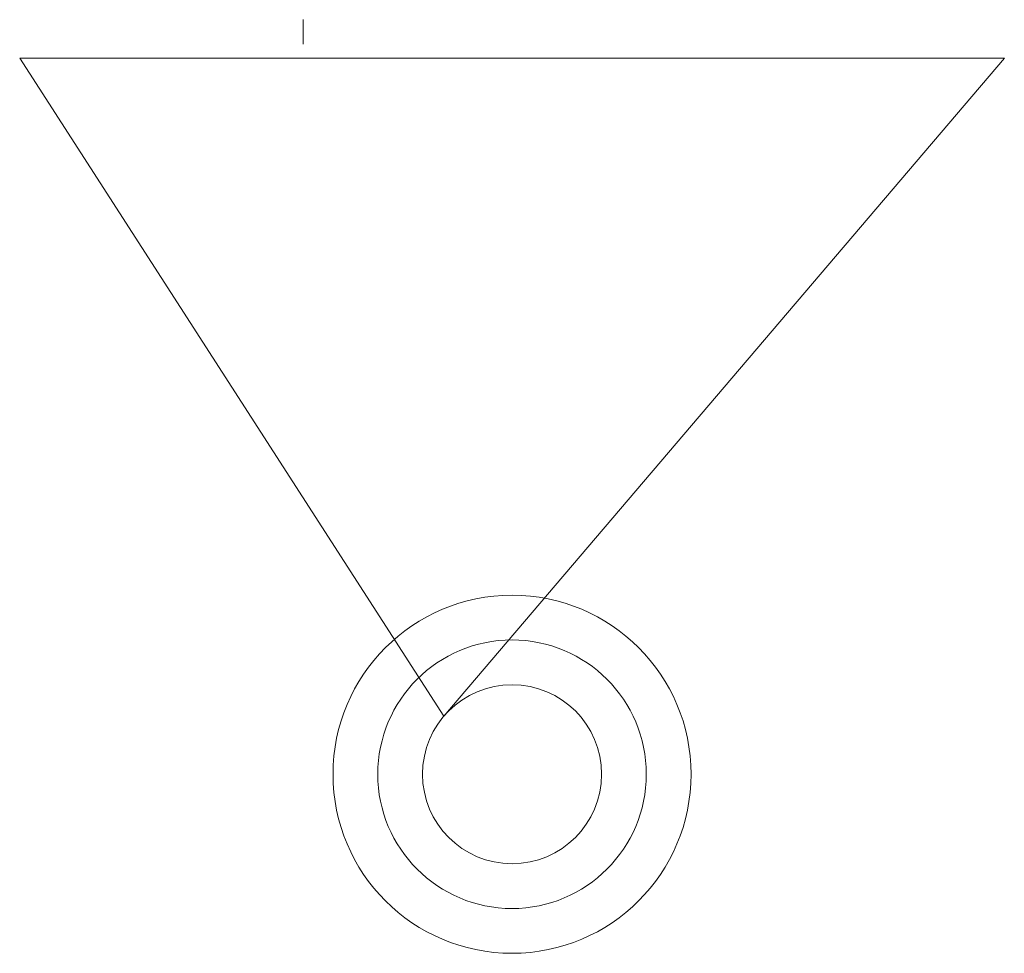
# Model space of a CAD drawing. Units: millimetres. Extents: x 0 to 3678, y 1592 to 1922.
# Tile 2 of 2: x 3568 to 3678, y 1592 to 1696. Entities that reach past the tile are written whole.
import ezdxf

# ---------------------------------------------------------------- set-up
doc = ezdxf.new("R2010")
doc.units = ezdxf.units.MM
doc.layers.add('M-CONS', color=8, linetype='Continuous', lineweight=18)

msp = doc.modelspace()

# ---------------------------------------------------------------- linework, layer by layer
at = {"layer": 'M-CONS', "extrusion": (-1e-16, 1, -1e-16)}
msp.add_line((3599.94, 1696.13, -3.9), (3599.94, 1693.39, -3.9), dxfattribs=at)
at = {"layer": 'M-CONS'}
msp.add_polyline3d([(3568.28, 1691.84, -42), (3678.28, 1691.84, -42), (3615.66, 1618.32, -47.44)], close=True, dxfattribs=at)
for radius in [20, 15, 10]:
    msp.add_circle((3623.28, 1611.84), radius, dxfattribs=at)

doc.saveas('drawing.dxf')
